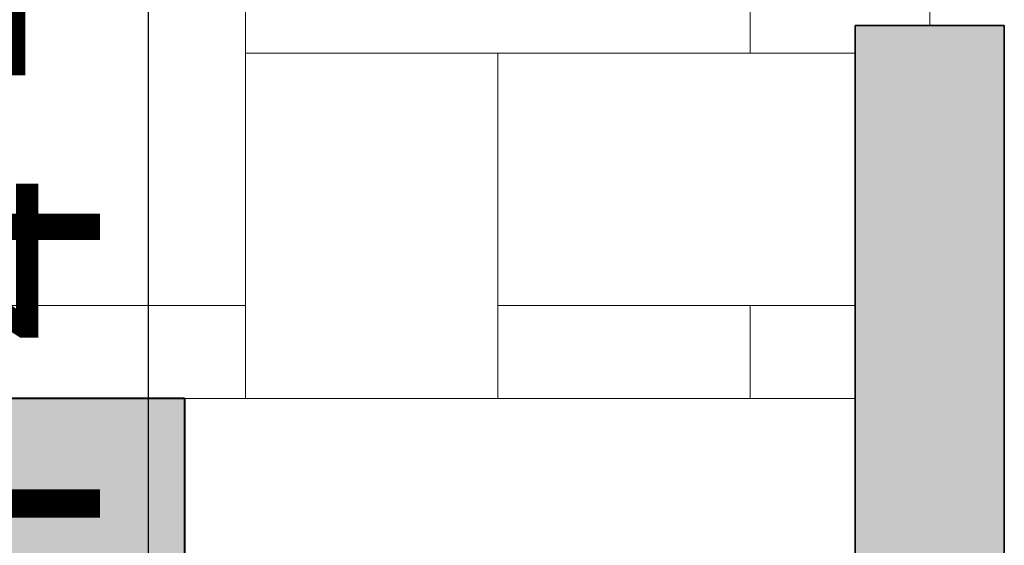
# Model space of a CAD drawing. Units: inches. Extents: x 2337 to 3570, y 1258 to 1938.
# Tile 17 of 30: x 2866 to 2906, y 1758 to 1779. Entities that reach past the tile are written whole.
import ezdxf

# ---------------------------------------------------------------- set-up
doc = ezdxf.new("R2010")
doc.units = ezdxf.units.IN
for name, color, linetype, lineweight in [('A-ANNO-DIMS', 2, 'Continuous', 18), ('A-FLOR-EDGE', 8, 'Continuous', 20), ('A-FLOR-PATT', 252, 'Continuous', 13), ('A-WALL', 7, 'Continuous', 40), ('C-PROP', 7, 'Continuous', 35), ('L-SITE-GATE', 4, 'Continuous', 18)]:
    doc.layers.add(name, color=color, linetype=linetype, lineweight=lineweight)
doc.layers.add('A-WALL-PATT', color=18, linetype='Continuous', lineweight=13, true_color=0x000000)
doc.layers.add('C-PROP-PATT', color=251, linetype='Continuous', lineweight=13, true_color=0x636466)
doc.styles.get("Standard").update_dxf_attribs({"font": 'arial.ttf'})
doc.dimstyles.new('ISO-25', dxfattribs={"dimtxt": 9, "dimasz": 2.5, "dimexe": 1.25, "dimexo": 0.625, "dimtad": 1, "dimdec": 1, "dimlunit": 3, "dimtxsty": 'Standard', "dimcen": 2.5, "dimadec": 0, "dimazin": 0, "dimtfac": 1, "dimtdec": 1, "dimtmove": 0, "dimatfit": 3, "dimfxl": 1, "dimarcsym": 0})

# ---------------------------------------------------------------- blocks, each defined once
blk = doc.blocks.new('*D90')
at = {"layer": 'A-ANNO-DIMS', "color": 0, "lineweight": -2, "transparency": 16777216}
for p, q in [((2871.382, 1676.497), (2871.382, 1796.695)), ((2864.515, 1676.497), (2872.632, 1676.497)), ((2871.382, 1629.048), (2871.382, 1673.997)), ((2864.515, 1626.548), (2872.632, 1626.548))]:
    blk.add_line(p, q, dxfattribs=at)
at = {"layer": 'A-ANNO-DIMS', "color": 0, "transparency": 16777216}
for points in [[(2870.966, 1673.997), (2871.799, 1673.997), (2871.382, 1676.497)], [(2870.966, 1629.048), (2871.799, 1629.048), (2871.382, 1626.548)]]:
    blk.add_solid(points, dxfattribs=at)
at = {"layer": 'Defpoints', "color": 0, "transparency": 16777216}
for p in [(2863.89, 1676.497), (2871.382, 1676.497), (2863.89, 1626.548)]:
    blk.add_point(p, dxfattribs=at)
at = {"layer": 'A-ANNO-DIMS', "color": 0, "transparency": 16777216, "insert": (2866.101, 1737.846), "char_height": 9, "attachment_point": 5, "rotation": 90}
blk.add_mtext('LOUNGE SEAT 4\'-2"', dxfattribs=at)

msp = doc.modelspace()

# ---------------------------------------------------------------- hatches: boundary and pattern name
at = {"layer": 'A-FLOR-PATT', "transparency": 33554687}
h = msp.add_hatch(dxfattribs=at)
h.set_pattern_fill('AR-HBONE', color=256, scale=0.1, angle=45)
h.paths.add_polyline_path([(2902.836, 1875.116), (2899.836, 1875.116), (2899.836, 1887.116), (2671.836, 1887.116), (2671.836, 1857.116), (2681.836, 1857.116), (2681.836, 1810.116), (2719.836, 1810.116), (2719.836, 1764.116), (2872.836, 1764.116), (2899.836, 1764.116), (2899.836, 1779.116), (2902.836, 1779.116)])
h.paths.add_polyline_path([(2854.179, 1832.557), (2857.321, 1832.422), (2861.942, 1831.206, -0.088302), (2868.629, 1828.111), (2871.77, 1825.918, -0.105467), (2873.266, 1824.315), (2874.966, 1823.992), (2877.339, 1822.551), (2875.419, 1827.303), (2873.36, 1826.955, -0.132795), (2873.22, 1833.505), (2876.098, 1833.321), (2876.098, 1832.971), (2877.275, 1832.476, -0.091085), (2878.864, 1831.436, -0.069602), (2881.45, 1828.175, -0.141553), (2886.249, 1809.409, -0.141553), (2881.487, 1790.635, -0.069602), (2878.907, 1787.369, -0.091085), (2877.321, 1786.326), (2876.14, 1785.827, -0.354729), (2875.735, 1785.451), (2873.268, 1785.288, -0.132795), (2873.395, 1791.839), (2875.455, 1791.495), (2877.365, 1796.25), (2874.995, 1794.805), (2873.296, 1794.479, -0.105467), (2871.802, 1792.873), (2868.666, 1790.673, -0.088302), (2861.985, 1787.565), (2857.366, 1786.339), (2854.225, 1786.199), (2827.803, 1783.011, -0.315912), (2819.634, 1782.954), (2793.542, 1785.741), (2798.79, 1786.943), (2825.847, 1785.283, 0.026512), (2832.53, 1785.227), (2857.366, 1786.339), (2861.985, 1787.565, 0.088302), (2868.666, 1790.673), (2871.802, 1792.873, 0.191215), (2873.932, 1796.114), (2875.792, 1805.131, 0.102572), (2875.784, 1813.667), (2873.906, 1822.681, 0.191215), (2871.77, 1825.918), (2868.629, 1828.111, 0.088302), (2861.942, 1831.206), (2857.321, 1832.422), (2832.483, 1833.486, 0.026512), (2825.799, 1833.417), (2798.745, 1831.704), (2793.496, 1832.895), (2819.582, 1835.733, -0.315912), (2827.751, 1835.692)], flags=16)
h.paths.add_polyline_path([(2862.34, 1826.572), (2867.3, 1825.996, -0.316515), (2870.308, 1823.311), (2872.444, 1814.149, -0.11452), (2872.453, 1804.643), (2870.336, 1795.477, -0.316515), (2867.333, 1792.786), (2862.374, 1792.2, -0.464922), (2861.397, 1793.116), (2861.861, 1801.965), (2861.836, 1809.385), (2861.846, 1816.806), (2861.365, 1825.654, -0.464922)], flags=16)
h.paths.add_polyline_path([(2821.293, 1791.09), (2807.573, 1791.499, -0.405226), (2805.023, 1794.123), (2805.023, 1794.121, 0.40508), (2807.573, 1791.499), (2821.293, 1791.09, 0.423258), (2823.999, 1793.719), (2823.999, 1793.719, -0.423258)], flags=16)
h.paths.add_polyline_path([(2879.429, 1814.798), (2881.737, 1813.816), (2882.582, 1811.673), (2882.717, 1809.406), (2882.586, 1807.139), (2881.746, 1804.994), (2879.439, 1804.008), (2880.042, 1807.699, 0.081616), (2880.039, 1811.108)], flags=0)
h.paths.add_polyline_path([(2796.957, 1829.715), (2796.14, 1815.428, 0.029076), (2796.152, 1803.213), (2796.997, 1788.928, -0.409057), (2796.19, 1788.002), (2791.055, 1787.607), (2785.763, 1792.935, -0.173254), (2784.26, 1796.136), (2783.472, 1804.33, -0.047466), (2783.462, 1814.286), (2784.234, 1822.482, -0.173254), (2785.73, 1825.686), (2791.012, 1831.024), (2796.148, 1830.639, -0.409057)], flags=16)
h.paths.add_polyline_path([(2750.344, 1835.795), (2750.012, 1834.37, 0.040009), (2748.771, 1826.064), (2748.631, 1824.022), (2750.526, 1825.239), (2756.614, 1827.237), (2771.951, 1829.419), (2781.401, 1831.049), (2780.099, 1822.888), (2779.438, 1814.328), (2779.144, 1809.304), (2779.447, 1804.281), (2780.126, 1795.721), (2781.444, 1787.563), (2771.99, 1789.174), (2756.65, 1791.337), (2750.557, 1793.323), (2748.66, 1794.536), (2748.804, 1792.494, 0.040009), (2750.062, 1784.191), (2750.396, 1782.767), (2745.899, 1784.642), (2744.102, 1788.129), (2743.099, 1791.925), (2741.068, 1802.995), (2740.859, 1809.271), (2741.055, 1815.548), (2743.065, 1826.622), (2744.061, 1830.421), (2745.851, 1833.911)], flags=16)
h.paths.add_polyline_path([(2761.183, 1831.202), (2754.851, 1829.51), (2754.556, 1830.832, -0.143032), (2754.62, 1831.812), (2755.053, 1833), (2761.169, 1831.713, -0.789416)], flags=16)
h.paths.add_polyline_path([(2761.226, 1787.381), (2754.89, 1789.061), (2754.599, 1787.738, 0.143032), (2754.665, 1786.758), (2755.1, 1785.571), (2761.213, 1786.87, 0.789416)], flags=16)
h.paths.add_polyline_path([(2689.028, 1816.171), (2701.274, 1816.171), (2701.274, 1823.798), (2689.028, 1823.798)], flags=24)
h.paths.add_polyline_path([(2755.384, 1858.953), (2808.715, 1858.953), (2808.715, 1885.073), (2755.384, 1885.073)], flags=24)
at = {"layer": 'A-WALL-PATT'}
h = msp.add_hatch(color=256, dxfattribs=at)
h.dxf.hatch_style = 1
h.paths.add_polyline_path([(2671.836, 1857.116), (2455.836, 1857.116), (2455.836, 1824.116), (2464.836, 1824.116), (2464.836, 1848.116), (2671.836, 1848.116)])
h.paths.add_polyline_path([(2566.836, 1764.116), (2464.836, 1764.116), (2464.836, 1788.116), (2455.836, 1788.116), (2455.836, 1743.116), (2464.836, 1743.116), (2464.836, 1755.116), (2566.836, 1755.116)])
h.paths.add_polyline_path([(2683.836, 1761.116), (2683.836, 1764.116), (2602.836, 1764.116), (2602.836, 1755.116), (2608.836, 1755.116), (2608.836, 1701.116), (2662.836, 1701.116), (2662.836, 1605.116), (2671.836, 1605.116), (2671.836, 1713.116), (2662.836, 1713.116), (2662.836, 1707.116), (2614.836, 1707.116), (2614.836, 1755.116), (2662.836, 1755.116), (2662.836, 1749.116), (2671.836, 1749.116), (2671.836, 1755.116), (2683.836, 1755.116)])
h.paths.add_polyline_path([(2464.836, 1707.116), (2455.836, 1707.116), (2455.836, 1617.116), (2464.836, 1617.116), (2464.836, 1635.116), (2506.836, 1635.116), (2506.836, 1641.116), (2464.836, 1641.116)])
h.paths.add_polyline_path([(2542.836, 1551.116), (2464.836, 1551.116), (2464.836, 1569.116), (2455.836, 1569.116), (2455.836, 1518.116), (2464.836, 1518.116), (2464.836, 1542.116), (2542.836, 1542.116)])
h.paths.add_polyline_path([(2464.836, 1482.116), (2455.836, 1482.116), (2455.836, 1410.116), (2464.836, 1410.116)])
h.paths.add_polyline_path([(2626.836, 1350.116), (2590.836, 1350.116), (2590.836, 1380.116), (2584.836, 1380.116), (2584.836, 1350.116), (2464.836, 1350.116), (2464.836, 1374.116), (2455.836, 1374.116), (2455.836, 1341.116), (2626.836, 1341.116)])
h.paths.add_polyline_path([(2662.836, 1416.116), (2686.836, 1416.116), (2686.836, 1422.116), (2590.836, 1422.116), (2590.836, 1542.116), (2680.836, 1542.116), (2680.836, 1551.116), (2671.836, 1551.116), (2671.836, 1557.116), (2662.836, 1557.116), (2662.836, 1551.116), (2578.836, 1551.116), (2578.836, 1542.116), (2584.836, 1542.116), (2584.836, 1410.116), (2590.836, 1410.116), (2590.836, 1416.116), (2656.836, 1416.116), (2656.836, 1350.116), (2650.836, 1350.116), (2650.836, 1341.116), (2731.836, 1341.116), (2731.836, 1362.116), (2722.836, 1362.116), (2722.836, 1350.116), (2662.836, 1350.116)])
h.paths.add_polyline_path([(2731.836, 1434.116), (2722.836, 1434.116), (2722.836, 1422.116), (2716.836, 1422.116), (2716.836, 1416.116), (2722.836, 1416.116), (2722.836, 1386.116), (2731.836, 1386.116)], flags=17)
h.paths.add_polyline_path([(2731.836, 1542.116), (2752.836, 1542.116), (2752.836, 1551.116), (2716.836, 1551.116), (2716.836, 1545.116), (2716.836, 1542.116), (2722.836, 1542.116), (2722.836, 1482.116), (2731.836, 1482.116)])
h.paths.add_polyline_path([(2809.836, 1551.116), (2788.836, 1551.116), (2788.836, 1542.116), (2809.836, 1542.116), (2809.836, 1548.116)])
h.paths.add_polyline_path([(2872.836, 1647.116), (2863.836, 1647.116), (2863.836, 1551.116), (2857.836, 1551.116), (2857.836, 1548.116), (2857.836, 1542.116), (2872.836, 1542.116)])
h.paths.add_polyline_path([(2872.836, 1764.116), (2827.836, 1764.116), (2827.836, 1755.116), (2863.836, 1755.116), (2863.836, 1719.116), (2872.836, 1719.116)])
h.paths.add_polyline_path([(2755.836, 1764.116), (2719.836, 1764.116), (2719.836, 1755.116), (2755.836, 1755.116)])
at = {"layer": 'C-PROP-PATT'}
h = msp.add_hatch(color=256, dxfattribs=at)
h.dxf.hatch_style = 1
h.paths.add_polyline_path([(2905.836, 1893.116), (2425.836, 1893.116), (2425.836, 1293.116), (2731.836, 1293.116), (2731.836, 1299.116), (2431.836, 1299.116), (2431.836, 1887.116), (2899.836, 1887.116), (2899.836, 1875.116), (2905.836, 1875.116)])
h.paths.add_polyline_path([(2845.836, 1299.116), (2827.836, 1299.116), (2827.836, 1293.116), (2845.836, 1293.116)], flags=17)
h.paths.add_polyline_path([(2905.836, 1779.116), (2899.836, 1779.116), (2899.836, 1299.116), (2893.836, 1299.116), (2893.836, 1293.116), (2905.836, 1293.116)], flags=17)

# ---------------------------------------------------------------- linework, layer by layer
at = {"layer": 'A-FLOR-EDGE'}
msp.add_line((2872.836, 1764.116), (2899.836, 1764.116), dxfattribs=at)
at = {"layer": 'A-WALL'}
for q in [(2719.836, 1764.116), (2872.836, 1542.116)]:
    msp.add_line((2872.836, 1764.116), q, dxfattribs=at)
at = {"layer": 'C-PROP'}
for p, q in [((2899.836, 1779.116), (2899.836, 1299.116)), ((2899.836, 1779.116), (2905.836, 1779.116)), ((2905.836, 1779.116), (2905.836, 1293.116))]:
    msp.add_line(p, q, dxfattribs=at)
at = {"layer": 'L-SITE-GATE'}
msp.add_line((2902.836, 1875.116), (2902.836, 1779.116), dxfattribs=at)

# ---------------------------------------------------------------- dimensions: what is measured, and where the dimension line sits
at = {"layer": 'A-ANNO-DIMS'}
dim = msp.add_linear_dim(base=(2871.382, 1676.497), p1=(2863.89, 1626.548), p2=(2863.89, 1676.497), angle=90, text='LOUNGE SEAT <>', dimstyle='ISO-25', override={"dimdec": 1, "dimlfac": 1, "dimrnd": 0, "dimzin": 1, "dimdsep": 46, "dimlunit": 4, "dimfrac": 2}, dxfattribs=at)
dim.commit()
dim.dimension.update_dxf_attribs({"geometry": '*D90', "text_midpoint": (2866.101, 1737.846)})

doc.saveas('drawing.dxf')
